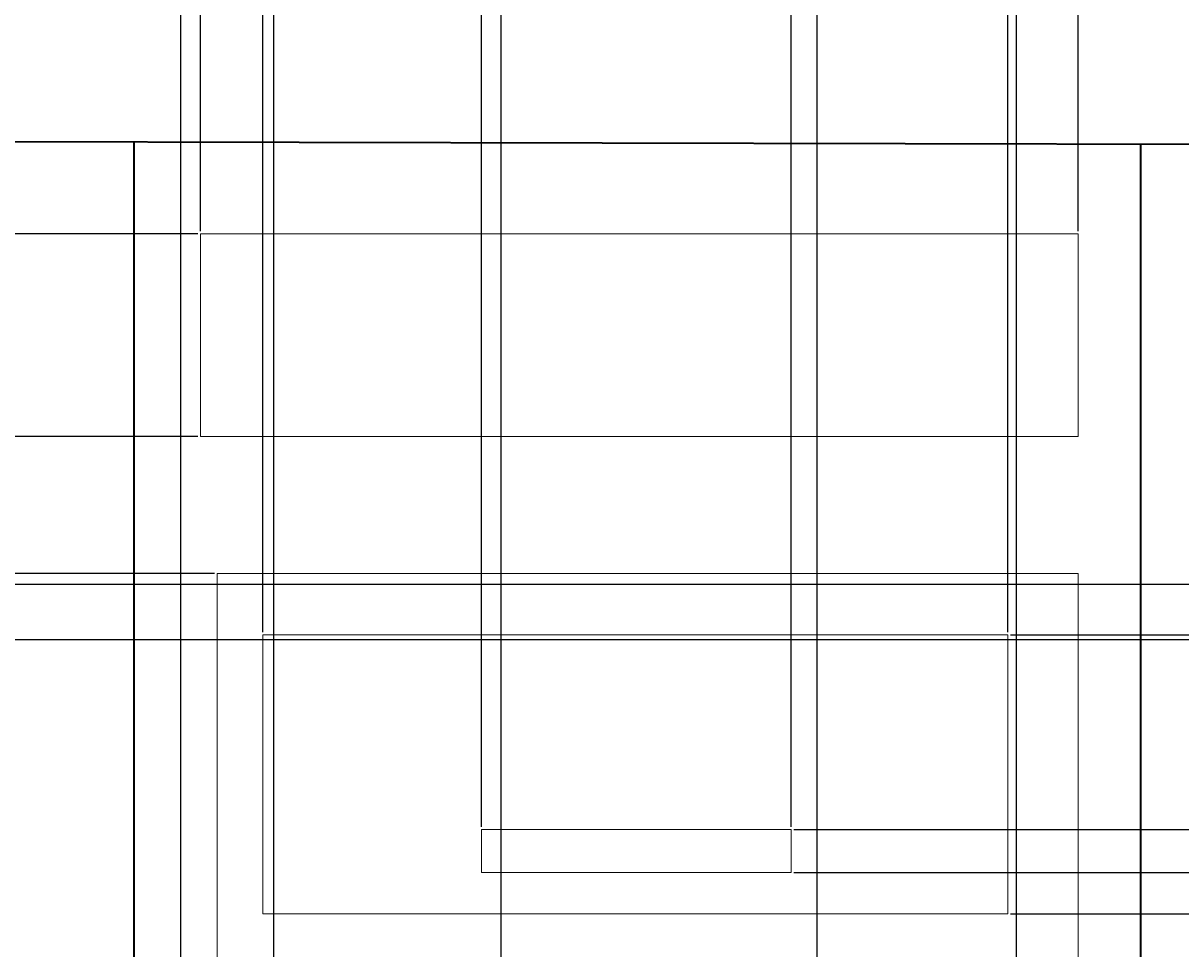
# Model space of a CAD drawing. Units: inches. Extents: x 27 to 200, y -50 to 102.
# Tile 11 of 26: x 117 to 144, y -3 to 19. Entities that reach past the tile are written whole.
import ezdxf

# ---------------------------------------------------------------- set-up
doc = ezdxf.new("R2010")
doc.units = ezdxf.units.IN
doc.header["$MEASUREMENT"] = 0
for name, color, linetype, lineweight in [('A-ANNO-DIMS', 2, 'Continuous', 18), ('A-ELEV', 7, 'Continuous', 35), ('A-FURN', 8, 'Continuous', 18)]:
    doc.layers.add(name, color=color, linetype=linetype, lineweight=lineweight)
doc.styles.get("Standard").update_dxf_attribs({"font": 'arial.ttf'})
doc.dimstyles.get("Standard").update_dxf_attribs({"dimtxt": 0.18, "dimasz": 0.18, "dimexe": 0.18, "dimexo": 0.0625, "dimgap": 0.09, "dimtad": 0, "dimtih": 1, "dimtoh": 1, "dimdec": 4, "dimzin": 0, "dimdsep": 46, "dimtxsty": 'Standard', "dimcen": 0.09, "dimadec": 0, "dimazin": 0, "dimtfac": 1, "dimtdec": 4, "dimtofl": 0, "dimtmove": 0, "dimatfit": 3, "dimfxl": 1, "dimtolj": 1, "dimtzin": 0, "dimarcsym": 0})

# ---------------------------------------------------------------- blocks, each defined once
blk = doc.blocks.new('*D48')
at = {"layer": 'A-ANNO-DIMS', "color": 0, "lineweight": -2, "transparency": 16777216}
for p, q in [((84.479, 44.926), (199.797, 44.926)), ((199.617, 44.746), (199.617, 14.26)), ((199.617, -16.589), (199.617, 13.897)), ((84.479, -16.769), (199.797, -16.769))]:
    blk.add_line(p, q, dxfattribs=at)
at = {"layer": 'A-ANNO-DIMS', "color": 0, "transparency": 16777216}
for points in [[(199.587, 44.746), (199.647, 44.746), (199.617, 44.926)], [(199.587, -16.589), (199.647, -16.589), (199.617, -16.769)]]:
    blk.add_solid(points, dxfattribs=at)
at = {"layer": 'Defpoints', "color": 0, "transparency": 16777216}
for p in [(84.417, 44.926), (199.617, 44.926), (84.417, -16.769)]:
    blk.add_point(p, dxfattribs=at)
at = {"layer": 'A-ANNO-DIMS', "color": 0, "transparency": 16777216, "insert": (199.617, 14.079), "char_height": 0.18, "attachment_point": 5}
blk.add_mtext('\\A1;61.7', dxfattribs=at)
blk = doc.blocks.new('*D51')
at = {"layer": 'A-ANNO-DIMS', "color": 0, "lineweight": -2, "transparency": 16777216}
for p, q in [((120.417, 45.561), (120.417, -25.149)), ((146.417, 45.561), (146.417, -25.149)), ((120.597, -24.969), (133.197, -24.969)), ((146.237, -24.969), (133.637, -24.969))]:
    blk.add_line(p, q, dxfattribs=at)
at = {"layer": 'A-ANNO-DIMS', "color": 0, "transparency": 16777216}
for points in [[(120.597, -24.939), (120.597, -24.999), (120.417, -24.969)], [(146.237, -24.939), (146.237, -24.999), (146.417, -24.969)]]:
    blk.add_solid(points, dxfattribs=at)
at = {"layer": 'Defpoints', "color": 0, "transparency": 16777216}
for p in [(120.417, 45.623), (146.417, 45.623), (146.417, -24.969)]:
    blk.add_point(p, dxfattribs=at)
at = {"layer": 'A-ANNO-DIMS', "color": 0, "transparency": 16777216, "insert": (133.417, -24.969), "char_height": 0.18, "attachment_point": 5}
blk.add_mtext('\\A1;26', dxfattribs=at)
blk = doc.blocks.new('*D53')
at = {"layer": 'A-ANNO-DIMS', "color": 0, "lineweight": -2, "transparency": 16777216}
for p, q in [((120.895, 14.04), (120.895, 102.306)), ((121.075, 102.126), (130.962, 102.126)), ((141.636, 102.126), (131.75, 102.126)), ((141.816, 14.04), (141.816, 102.306))]:
    blk.add_line(p, q, dxfattribs=at)
at = {"layer": 'A-ANNO-DIMS', "color": 0, "transparency": 16777216}
for points in [[(121.075, 102.156), (121.075, 102.096), (120.895, 102.126)], [(141.636, 102.156), (141.636, 102.096), (141.816, 102.126)]]:
    blk.add_solid(points, dxfattribs=at)
at = {"layer": 'Defpoints', "color": 0, "transparency": 16777216}
for p in [(141.816, 102.126), (120.895, 13.977), (141.816, 13.977)]:
    blk.add_point(p, dxfattribs=at)
at = {"layer": 'A-ANNO-DIMS', "color": 0, "transparency": 16777216, "insert": (131.356, 102.126), "char_height": 0.18, "attachment_point": 5}
blk.add_mtext('\\A1;20.92', dxfattribs=at)
blk = doc.blocks.new('*D54')
at = {"layer": 'A-ANNO-DIMS', "color": 0, "lineweight": -2, "transparency": 16777216}
for p, q in [((120.833, 13.977), (27.037, 13.977)), ((27.217, 13.797), (27.217, 11.743)), ((27.217, 9.324), (27.217, 11.379)), ((120.833, 9.144), (27.037, 9.144))]:
    blk.add_line(p, q, dxfattribs=at)
at = {"layer": 'A-ANNO-DIMS', "color": 0, "transparency": 16777216}
for points in [[(27.187, 13.797), (27.247, 13.797), (27.217, 13.977)], [(27.187, 9.324), (27.247, 9.324), (27.217, 9.144)]]:
    blk.add_solid(points, dxfattribs=at)
at = {"layer": 'Defpoints', "color": 0, "transparency": 16777216}
for p in [(27.217, 13.977), (120.895, 13.977), (120.895, 9.144)]:
    blk.add_point(p, dxfattribs=at)
at = {"layer": 'A-ANNO-DIMS', "color": 0, "transparency": 16777216, "insert": (27.217, 11.561), "char_height": 0.18, "attachment_point": 5}
blk.add_mtext('\\A1;4.83', dxfattribs=at)
blk = doc.blocks.new('*D56')
at = {"layer": 'A-ANNO-DIMS', "color": 0, "lineweight": -2, "transparency": 16777216}
for p, q in [((121.225, 5.878), (27.037, 5.878)), ((27.217, 5.698), (27.217, -3.085)), ((27.217, -12.231), (27.217, -3.448)), ((121.225, -12.411), (27.037, -12.411))]:
    blk.add_line(p, q, dxfattribs=at)
at = {"layer": 'A-ANNO-DIMS', "color": 0, "transparency": 16777216}
for points in [[(27.187, 5.698), (27.247, 5.698), (27.217, 5.878)], [(27.187, -12.231), (27.247, -12.231), (27.217, -12.411)]]:
    blk.add_solid(points, dxfattribs=at)
at = {"layer": 'Defpoints', "color": 0, "transparency": 16777216}
for p in [(27.217, 5.878), (121.288, 5.878), (121.288, -12.411)]:
    blk.add_point(p, dxfattribs=at)
at = {"layer": 'A-ANNO-DIMS', "color": 0, "transparency": 16777216, "insert": (27.217, -3.267), "char_height": 0.18, "attachment_point": 5}
blk.add_mtext('\\A1;18.29', dxfattribs=at)
blk = doc.blocks.new('*D57')
at = {"layer": 'A-ANNO-DIMS', "color": 0, "lineweight": -2, "transparency": 16777216}
for p, q in [((122.38, 4.48), (122.38, 102.306)), ((122.56, 102.126), (130.875, 102.126)), ((139.961, 102.126), (131.645, 102.126)), ((140.141, 4.48), (140.141, 102.306))]:
    blk.add_line(p, q, dxfattribs=at)
at = {"layer": 'A-ANNO-DIMS', "color": 0, "transparency": 16777216}
for points in [[(122.56, 102.156), (122.56, 102.096), (122.38, 102.126)], [(139.961, 102.156), (139.961, 102.096), (140.141, 102.126)]]:
    blk.add_solid(points, dxfattribs=at)
at = {"layer": 'Defpoints', "color": 0, "transparency": 16777216}
for p in [(140.141, 102.126), (122.38, 4.418), (140.141, 4.418)]:
    blk.add_point(p, dxfattribs=at)
at = {"layer": 'A-ANNO-DIMS', "color": 0, "transparency": 16777216, "insert": (131.26, 102.126), "char_height": 0.18, "attachment_point": 5}
blk.add_mtext('\\A1;17.76', dxfattribs=at)
blk = doc.blocks.new('*D58')
at = {"layer": 'A-ANNO-DIMS', "color": 0, "lineweight": -2, "transparency": 16777216}
for p, q in [((140.203, 4.418), (199.797, 4.418)), ((199.617, 4.238), (199.617, 1.273)), ((199.617, -2.056), (199.617, 0.909)), ((140.203, -2.236), (199.797, -2.236))]:
    blk.add_line(p, q, dxfattribs=at)
at = {"layer": 'A-ANNO-DIMS', "color": 0, "transparency": 16777216}
for points in [[(199.587, 4.238), (199.647, 4.238), (199.617, 4.418)], [(199.587, -2.056), (199.647, -2.056), (199.617, -2.236)]]:
    blk.add_solid(points, dxfattribs=at)
at = {"layer": 'Defpoints', "color": 0, "transparency": 16777216}
for p in [(140.141, 4.418), (199.617, 4.418), (140.141, -2.236)]:
    blk.add_point(p, dxfattribs=at)
at = {"layer": 'A-ANNO-DIMS', "color": 0, "transparency": 16777216, "insert": (199.617, 1.091), "char_height": 0.18, "attachment_point": 5}
blk.add_mtext('\\A1;6.654', dxfattribs=at)
blk = doc.blocks.new('*D59')
at = {"layer": 'A-ANNO-DIMS', "color": 0, "lineweight": -2, "transparency": 16777216}
for p, q in [((127.595, -0.162), (127.595, 102.306)), ((127.775, 102.126), (130.893, 102.126)), ((134.798, 102.126), (131.679, 102.126)), ((134.978, -0.162), (134.978, 102.306))]:
    blk.add_line(p, q, dxfattribs=at)
at = {"layer": 'A-ANNO-DIMS', "color": 0, "transparency": 16777216}
for points in [[(127.775, 102.156), (127.775, 102.096), (127.595, 102.126)], [(134.798, 102.156), (134.798, 102.096), (134.978, 102.126)]]:
    blk.add_solid(points, dxfattribs=at)
at = {"layer": 'Defpoints', "color": 0, "transparency": 16777216}
for p in [(134.978, 102.126), (127.595, -0.225), (134.978, -0.225)]:
    blk.add_point(p, dxfattribs=at)
at = {"layer": 'A-ANNO-DIMS', "color": 0, "transparency": 16777216, "insert": (131.286, 102.126), "char_height": 0.18, "attachment_point": 5}
blk.add_mtext('\\A1;7.383', dxfattribs=at)
blk = doc.blocks.new('*D60')
at = {"layer": 'A-ANNO-DIMS', "color": 0, "lineweight": -2, "transparency": 16777216}
for p, q in [((135.04, -0.225), (199.797, -0.225)), ((199.617, -0.405), (199.617, -0.559)), ((199.617, -1.076), (199.617, -0.923)), ((135.04, -1.256), (199.797, -1.256))]:
    blk.add_line(p, q, dxfattribs=at)
at = {"layer": 'A-ANNO-DIMS', "color": 0, "transparency": 16777216}
for points in [[(199.587, -0.405), (199.647, -0.405), (199.617, -0.225)], [(199.587, -1.076), (199.647, -1.076), (199.617, -1.256)]]:
    blk.add_solid(points, dxfattribs=at)
at = {"layer": 'Defpoints', "color": 0, "transparency": 16777216}
for p in [(134.978, -0.225), (199.617, -0.225), (134.978, -1.256)]:
    blk.add_point(p, dxfattribs=at)
at = {"layer": 'A-ANNO-DIMS', "color": 0, "transparency": 16777216, "insert": (199.617, -0.741), "char_height": 0.18, "attachment_point": 5}
blk.add_mtext('\\A1;1.03', dxfattribs=at)
blk = doc.blocks.new('*D61')
at = {"layer": 'A-ANNO-DIMS', "color": 0, "lineweight": -2, "transparency": 16777216}
for p, q in [((122.638, -4.237), (122.638, 102.306)), ((122.818, 102.126), (131.125, 102.126)), ((140.167, 102.126), (131.86, 102.126)), ((140.347, -4.237), (140.347, 102.306))]:
    blk.add_line(p, q, dxfattribs=at)
at = {"layer": 'A-ANNO-DIMS', "color": 0, "transparency": 16777216}
for points in [[(122.818, 102.156), (122.818, 102.096), (122.638, 102.126)], [(140.167, 102.156), (140.167, 102.096), (140.347, 102.126)]]:
    blk.add_solid(points, dxfattribs=at)
at = {"layer": 'Defpoints', "color": 0, "transparency": 16777216}
for p in [(140.347, 102.126), (122.638, -4.3), (140.347, -4.3)]:
    blk.add_point(p, dxfattribs=at)
at = {"layer": 'A-ANNO-DIMS', "color": 0, "transparency": 16777216, "insert": (131.493, 102.126), "char_height": 0.18, "attachment_point": 5}
blk.add_mtext('\\A1;17.71', dxfattribs=at)
blk = doc.blocks.new('*D63')
at = {"layer": 'A-ANNO-DIMS', "color": 0, "lineweight": -2, "transparency": 16777216}
for p, q in [((128.059, -9.034), (128.059, 102.306)), ((128.239, 102.126), (131.435, 102.126)), ((135.417, 102.126), (132.221, 102.126)), ((135.597, -9.034), (135.597, 102.306))]:
    blk.add_line(p, q, dxfattribs=at)
at = {"layer": 'A-ANNO-DIMS', "color": 0, "transparency": 16777216}
for points in [[(128.239, 102.156), (128.239, 102.096), (128.059, 102.126)], [(135.417, 102.156), (135.417, 102.096), (135.597, 102.126)]]:
    blk.add_solid(points, dxfattribs=at)
at = {"layer": 'Defpoints', "color": 0, "transparency": 16777216}
for p in [(135.597, 102.126), (128.059, -9.097), (135.597, -9.097)]:
    blk.add_point(p, dxfattribs=at)
at = {"layer": 'A-ANNO-DIMS', "color": 0, "transparency": 16777216, "insert": (131.828, 102.126), "char_height": 0.18, "attachment_point": 5}
blk.add_mtext('\\A1;7.538', dxfattribs=at)
blk = doc.blocks.new('*D68')
at = {"layer": 'A-ANNO-DIMS', "color": 0, "lineweight": -2, "transparency": 16777216}
for p, q in [((145.153, 5.617), (27.037, 5.617)), ((27.217, 5.437), (27.217, 5.138)), ((27.217, 4.476), (27.217, 4.774)), ((145.153, 4.296), (27.037, 4.296))]:
    blk.add_line(p, q, dxfattribs=at)
at = {"layer": 'A-ANNO-DIMS', "color": 0, "transparency": 16777216}
for points in [[(27.187, 5.437), (27.247, 5.437), (27.217, 5.617)], [(27.187, 4.476), (27.247, 4.476), (27.217, 4.296)]]:
    blk.add_solid(points, dxfattribs=at)
at = {"layer": 'Defpoints', "color": 0, "transparency": 16777216}
for p in [(27.217, 5.617), (145.216, 5.617), (145.216, 4.296)]:
    blk.add_point(p, dxfattribs=at)
at = {"layer": 'A-ANNO-DIMS', "color": 0, "transparency": 16777216, "insert": (27.217, 4.956), "char_height": 0.18, "attachment_point": 5}
blk.add_mtext('\\A1;1.32', dxfattribs=at)

msp = doc.modelspace()

# ---------------------------------------------------------------- linework, layer by layer
at = {"layer": 'A-ELEV'}
for p, q in [((191.4102, 16.002), (89.3051, 16.2307)), ((119.3118, -16.7693), (119.3118, 16.1635)), ((143.3118, -16.7693), (143.3118, 16.1097))]:
    msp.add_line(p, q, dxfattribs=at)
at = {"layer": 'A-FURN'}
for points in [[(120.8954, 13.9773), (141.8163, 13.9773), (141.8163, 9.1438), (120.8954, 9.1438)], [(121.2876, 5.8779), (141.8163, 5.8779), (141.8163, -12.411), (121.2876, -12.411)], [(122.38, 4.4177), (140.1406, 4.4177), (140.1406, -2.2364), (122.38, -2.2364)], [(127.5946, -0.2247), (134.9776, -0.2247), (134.9776, -1.2564), (127.5946, -1.2564)]]:
    msp.add_lwpolyline(points, close=True, dxfattribs=at)

# ---------------------------------------------------------------- dimensions: what is measured, and where the dimension line sits
at = {"layer": 'A-ANNO-DIMS'}
for base, p1, p2, override, picture, middle in [((141.8163, 102.1264), (120.8954, 13.9773), (141.8163, 13.9773), {"dimdec": 2, "dimlfac": 1, "dimrnd": 0, "dimzin": 0, "dimdsep": 46, "dimlunit": 2}, '*D53', (131.3558, 102.1264)), ((140.1406, 102.1264), (122.38, 4.4177), (140.1406, 4.4177), {"dimdec": 2, "dimlfac": 1, "dimrnd": 0, "dimzin": 0, "dimdsep": 46, "dimlunit": 2}, '*D57', (131.2603, 102.1264)), ((140.3471, 102.1264), (122.6381, -4.2997), (140.3471, -4.2997), {"dimdec": 2, "dimlfac": 1, "dimrnd": 0, "dimzin": 0, "dimdsep": 46, "dimlunit": 2}, '*D61', (131.4926, 102.1264)), ((134.9776, 102.1264), (127.5946, -0.2247), (134.9776, -0.2247), {"dimdec": 3, "dimlfac": 1, "dimrnd": 0, "dimzin": 0, "dimdsep": 46, "dimlunit": 2}, '*D59', (131.2861, 102.1264)), ((135.5972, 102.1264), (128.0592, -9.0968), (135.5972, -9.0968), {"dimdec": 3, "dimlfac": 1, "dimrnd": 0, "dimzin": 0, "dimdsep": 46, "dimlunit": 2}, '*D63', (131.8282, 102.1264)), ((146.4169, -24.9693), (120.4169, 45.6231), (146.4169, 45.6231), {"dimdec": 0, "dimlfac": 1, "dimrnd": 0, "dimzin": 0, "dimdsep": 46, "dimlunit": 2}, '*D51', (133.4169, -24.9693))]:
    dim = msp.add_linear_dim(base=base, p1=p1, p2=p2, dimstyle='Standard', override=override, dxfattribs=at)
    dim.commit()
    dim.dimension.update_dxf_attribs({"geometry": picture, "text_midpoint": middle})
for base, p1, p2, override, picture, middle in [((199.6169, 44.9264), (84.4169, -16.7693), (84.4169, 44.9264), {"dimdec": 1, "dimlfac": 1, "dimrnd": 0, "dimzin": 0, "dimdsep": 46, "dimlunit": 2}, '*D48', (199.6169, 14.0786)), ((27.2169, 13.9773), (120.8954, 9.1438), (120.8954, 13.9773), {"dimdec": 2, "dimlfac": 1, "dimrnd": 0, "dimzin": 0, "dimdsep": 46, "dimlunit": 2}, '*D54', (27.2169, 11.5606)), ((27.2169, 5.8779), (121.2876, -12.411), (121.2876, 5.8779), {"dimdec": 2, "dimlfac": 1, "dimrnd": 0, "dimzin": 0, "dimdsep": 46, "dimlunit": 2}, '*D56', (27.2169, -3.2665)), ((27.2169, 5.6167), (145.216, 4.2959), (145.216, 5.6167), {"dimdec": 2, "dimlfac": 1, "dimrnd": 0, "dimzin": 0, "dimdsep": 46, "dimlunit": 2}, '*D68', (27.2169, 4.9563)), ((199.6169, 4.4177), (140.1406, -2.2364), (140.1406, 4.4177), {"dimdec": 3, "dimlfac": 1, "dimrnd": 0, "dimzin": 0, "dimdsep": 46, "dimlunit": 2}, '*D58', (199.6169, 1.0906)), ((199.6169, -0.2247), (134.9776, -1.2564), (134.9776, -0.2247), {"dimdec": 2, "dimlfac": 1, "dimrnd": 0, "dimzin": 0, "dimdsep": 46, "dimlunit": 2}, '*D60', (199.6169, -0.7405))]:
    dim = msp.add_linear_dim(base=base, p1=p1, p2=p2, angle=90, dimstyle='Standard', override=override, dxfattribs=at)
    dim.commit()
    dim.dimension.update_dxf_attribs({"geometry": picture, "text_midpoint": middle})

doc.saveas('drawing.dxf')
